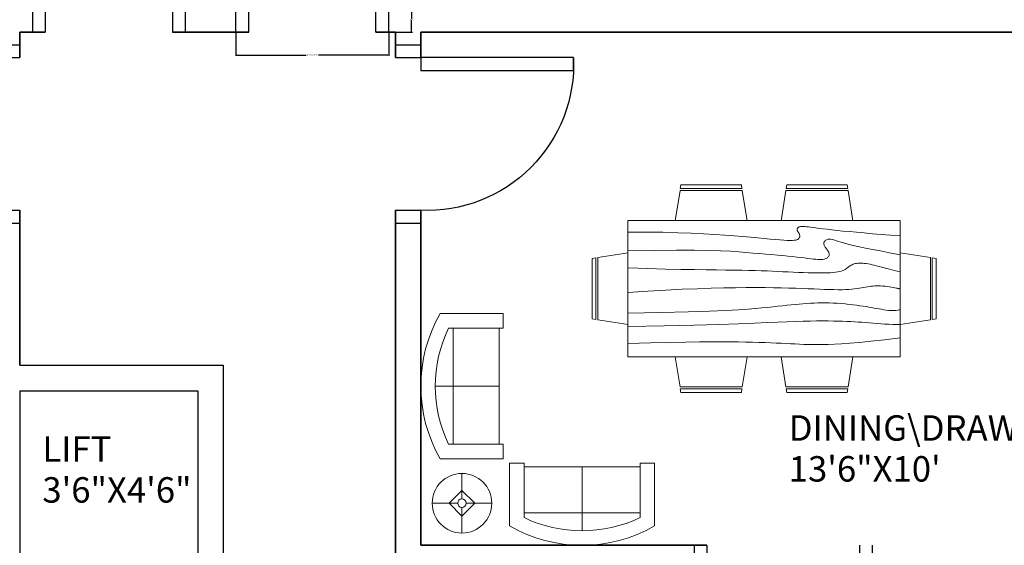
# Model space of a CAD drawing. Units: inches. Extents: x 4159 to 4826, y 299 to 1026.
# Tile 33 of 37: x 4453 to 4685, y 539 to 663. Entities that reach past the tile are written whole.
import ezdxf

# ---------------------------------------------------------------- set-up
doc = ezdxf.new("R2010")
doc.units = ezdxf.units.IN
for name, color, linetype, lineweight in [('A-ANNO-DIMS', 2, 'Continuous', 18), ('A-AREA-IDEN', 7, 'Continuous', 18), ('A-DOOR', 4, 'Continuous', 25), ('A-FLOR-EVTR', 6, 'Continuous', 25), ('A-FURN', 8, 'Continuous', 18), ('A-WALL', 7, 'Continuous', 35)]:
    doc.layers.add(name, color=color, linetype=linetype, lineweight=lineweight)
doc.styles.get("Standard").update_dxf_attribs({"font": 'arial.ttf'})
doc.dimstyles.get("Standard").update_dxf_attribs({"dimtxt": 0.18, "dimasz": 0.18, "dimexe": 0.18, "dimexo": 0.0625, "dimgap": 0.09, "dimtad": 0, "dimtih": 1, "dimtoh": 1, "dimdec": 4, "dimzin": 0, "dimdsep": 46, "dimtxsty": 'Standard', "dimcen": 0.09, "dimadec": 0, "dimazin": 0, "dimtfac": 1, "dimtdec": 4, "dimtofl": 0, "dimtmove": 0, "dimatfit": 3, "dimfxl": 1, "dimtolj": 1, "dimtzin": 0, "dimarcsym": 0})

# ---------------------------------------------------------------- blocks, each defined once
blk = doc.blocks.new('Sofa - Roundback Loveseat 5 ft.')
for p, q in [((0, -32.44198), (0, -5.99998)), ((-24, -33.99998), (-24, -11.46958)), ((24.00004, -33.99998), (24.00004, -11.46958)), ((-23.9998, -13.38178), (23.99986, -13.38178)), ((-24, -32.44198), (24.00004, -32.44198))]:
    blk.add_line(p, q)
for points in [[(-24, -33.99998), (-30, -33.99998), (-30, -7.99998)], [(30.00004, -7.99998), (30.00004, -33.99998), (24.00004, -33.99998)]]:
    blk.add_lwpolyline(points)
for centre, radius, start, end in [((0, -60.24998), 60.24998, 60.13715, 119.8628), ((0, -61.38438), 55.38444, 64.32083, 115.6792)]:
    blk.add_arc(centre, radius, start, end)
blk = doc.blocks.new('Dining Set - 36 x 72 in.')
for p, q in [((-22, 27.5), (-22.1562, 26.50042)), ((-5.8416, 26.5), (-22.1534, 26.5)), ((-22, 27.5), (-6, 27.5)), ((-5.8437, 26.49966), (-6, 27.5)), ((6, 27.5), (5.8438, 26.50042)), ((22.1584, 26.5), (5.8466, 26.5)), ((6, 27.5), (22, 27.5)), ((22.1563, 26.49966), (22, 27.5)), ((-22.2343, 26.00059), (-23.4847, 17.99762)), ((-22.2304, 26), (-5.7608, 26)), ((-4.5152, 17.99762), (-5.7655, 25.99926)), ((5.7657, 26.00059), (4.5153, 17.99762)), ((5.7696, 26), (22.2392, 26)), ((23.4848, 17.99762), (22.2345, 25.99926)), ((36, 18), (-36, 18)), ((-36, 18), (-36, -18)), ((36, -18), (36, 18)), ((-45.5, 8), (-44.5004, 8.15617)), ((-45.5, 8), (-45.5, -8)), ((-44.5, -8.15843), (-44.5, 8.15338)), ((-44.0006, 8.23428), (-35.9976, 9.48474)), ((-44, 8.23041), (-44, -8.23915)), ((44.0006, 8.23428), (35.9976, 9.48474)), ((44, 8.23041), (44, -8.23915)), ((44.5, -8.15843), (44.5, 8.15338)), ((45.5, 8), (44.5005, 8.15617)), ((45.5, 8), (45.5, -8)), ((-44.4997, -8.15631), (-45.5, -8)), ((-35.9976, -9.48476), (-43.9993, -8.2345)), ((35.9976, -9.48476), (43.9993, -8.2345)), ((44.4997, -8.15631), (45.5, -8)), ((-36, -18), (36, -18)), ((-22.2343, -26.0006), (-23.4847, -17.99762)), ((-4.5152, -17.99762), (-5.7655, -25.99928)), ((5.7657, -26.0006), (4.5153, -17.99762)), ((23.4848, -17.99762), (22.2345, -25.99928)), ((-22.2304, -26), (-5.7608, -26)), ((5.7696, -26), (22.2392, -26)), ((-22, -27.5), (-22.1562, -26.50044)), ((-5.8416, -26.5), (-22.1534, -26.5)), ((-22, -27.5), (-6, -27.5)), ((-5.8437, -26.49967), (-6, -27.5)), ((6, -27.5), (5.8438, -26.50044)), ((22.1584, -26.5), (5.8466, -26.5)), ((6, -27.5), (22, -27.5)), ((22.1563, -26.49967), (22, -27.5))]:
    blk.add_line(p, q)
for points in [[(-36, 15), (-31.1772, 14.97754), (-26.8079, 14.91406), (-22.8538, 14.81543), (-19.276, 14.6875), (-16.0362, 14.53613), (-13.0957, 14.36718), (-10.4159, 14.18652), (-7.9583, 14), (-5.6904, 13.81315), (-3.6035, 13.63021), (-1.6954, 13.45508), (0.0365, 13.29166), (1.5945, 13.14388), (2.9811, 13.01562), (4.1988, 12.9108), (5.25, 12.83333), (6.1393, 12.78613), (6.8802, 12.76823), (7.4883, 12.77767), (7.9792, 12.8125), (8.3685, 12.87077), (8.6719, 12.95052), (8.9049, 13.0498), (9.0833, 13.16666), (9.2205, 13.29899), (9.3216, 13.44401), (9.3895, 13.59879), (9.4271, 13.76041), (9.4373, 13.92594), (9.4232, 14.09245), (9.3875, 14.257), (9.3333, 14.41666), (9.2638, 14.56917), (9.1836, 14.71484), (9.0975, 14.85465), (9.0104, 14.98958), (8.9272, 15.1206), (8.8529, 15.2487), (8.7922, 15.37483), (8.75, 15.5), (8.7305, 15.62467), (8.7344, 15.74739), (8.7617, 15.86621), (8.8125, 15.97916), (8.8867, 16.08431), (8.9844, 16.17968), (9.1055, 16.26334), (9.25, 16.33333), (9.4189, 16.38802), (9.6172, 16.42708), (9.8506, 16.45052), (10.125, 16.45833), (10.4463, 16.45052), (10.8203, 16.42708), (11.2529, 16.38802), (11.75, 16.33333), (12.3184, 16.26318), (12.9694, 16.17838), (13.7151, 16.07991), (14.5677, 15.96875), (15.5395, 15.84586), (16.6426, 15.71224), (17.8893, 15.56884), (19.2917, 15.41666), (20.859, 15.25667), (22.5879, 15.08984), (24.4721, 14.91715), (26.5052, 14.73958), (28.6809, 14.5581), (30.9929, 14.3737), (33.4347, 14.18733), (36, 14)], [(-36, 10), (-28.9766, 10.14274), (-23.1725, 10.20442), (-18.4241, 10.19775), (-14.5677, 10.13541), (-11.4399, 10.03011), (-8.877, 9.89453), (-6.7154, 9.74137), (-4.7917, 9.58333), (-2.9698, 9.43082), (-1.2246, 9.28515), (0.4415, 9.14534), (2.026, 9.01041), (3.5266, 8.87939), (4.9408, 8.7513), (6.266, 8.62516), (7.5, 8.5), (8.6411, 8.37549), (9.6914, 8.2539), (10.6538, 8.13818), (11.5312, 8.03125), (12.3267, 7.93603), (13.043, 7.85547), (13.6831, 7.79248), (14.25, 7.75), (14.7471, 7.7303), (15.1797, 7.73307), (15.5537, 7.75732), (15.875, 7.80208), (16.1494, 7.86637), (16.3828, 7.94922), (16.5811, 8.04964), (16.75, 8.16666), (16.8944, 8.29915), (17.0143, 8.44531), (17.1089, 8.60319), (17.1771, 8.77083), (17.218, 8.94629), (17.2305, 9.1276), (17.2137, 9.31282), (17.1667, 9.5), (17.0895, 9.6875), (16.987, 9.875), (16.8649, 10.0625), (16.7292, 10.25), (16.5856, 10.4375), (16.4401, 10.625), (16.2985, 10.8125), (16.1667, 11), (16.05, 11.18733), (15.9518, 11.3737), (15.8752, 11.5581), (15.8229, 11.73958), (15.798, 11.91715), (15.8034, 12.08984), (15.842, 12.25667), (15.9167, 12.41666), (16.0295, 12.56836), (16.1784, 12.70833), (16.3605, 12.83268), (16.5729, 12.9375), (16.8127, 13.01888), (17.0768, 13.07291), (17.3625, 13.0957), (17.6667, 13.08333), (17.9894, 13.03312), (18.3418, 12.94726), (18.7382, 12.82918), (19.1927, 12.68229), (19.7195, 12.51001), (20.3327, 12.31575), (21.0465, 12.10294), (21.875, 11.875), (22.8357, 11.63354), (23.959, 11.37304), (25.2786, 11.08618), (26.8282, 10.76562), (28.6414, 10.40405), (30.752, 9.99414), (33.1936, 9.52856), (36, 9)], [(-36, 5.5), (-30.7157, 5.3348), (-26.069, 5.20963), (-21.9946, 5.11767), (-18.4271, 5.05208), (-15.3009, 5.00602), (-12.5508, 4.97265), (-10.1112, 4.94515), (-7.9167, 4.91666), (-5.909, 4.88167), (-4.0586, 4.83984), (-2.3429, 4.79215), (-0.7396, 4.73958), (0.7739, 4.6831), (2.22, 4.6237), (3.6213, 4.56233), (5, 4.5), (6.373, 4.43782), (7.7344, 4.3776), (9.0723, 4.32129), (10.375, 4.27083), (11.6309, 4.22819), (12.8281, 4.19531), (13.9551, 4.17415), (15, 4.16666), (15.954, 4.17448), (16.819, 4.19791), (17.6001, 4.23698), (18.3021, 4.29166), (18.9299, 4.36198), (19.4883, 4.44791), (19.9823, 4.54948), (20.4167, 4.66666), (20.7969, 4.79899), (21.1302, 4.94401), (21.4245, 5.09879), (21.6875, 5.26041), (21.9271, 5.42594), (22.1511, 5.59245), (22.3672, 5.757), (22.5834, 5.91666), (22.8065, 6.06868), (23.0404, 6.21093), (23.2879, 6.34147), (23.5521, 6.45833), (23.8358, 6.55957), (24.142, 6.64323), (24.4735, 6.70735), (24.8334, 6.75), (25.2235, 6.76969), (25.642, 6.76692), (26.0858, 6.74267), (26.5521, 6.69791), (27.0379, 6.63362), (27.5404, 6.55078), (28.0565, 6.45036), (28.5834, 6.33333), (29.1242, 6.19987), (29.7071, 6.04687), (30.3661, 5.87044), (31.1354, 5.66666), (32.0493, 5.43164), (33.142, 5.16146), (34.4475, 4.85221), (36, 4.5)], [(-36, -1), (-30.7915, -0.6591), (-26.0195, -0.38216), (-21.6519, -0.16284), (-17.6563, 0.00521), (-14.0005, 0.12833), (-10.6523, 0.21289), (-7.5796, 0.26522), (-4.75, 0.29166), (-2.134, 0.29793), (0.2878, 0.28711), (2.5317, 0.26163), (4.6146, 0.22396), (6.5529, 0.17651), (8.3633, 0.12174), (10.0623, 0.06209), (11.6667, 0), (13.1899, -0.06201), (14.6341, -0.1211), (15.9982, -0.17432), (17.2813, -0.21875), (18.4823, -0.25147), (19.6003, -0.26953), (20.6343, -0.27002), (21.5834, -0.25), (22.4481, -0.20768), (23.2357, -0.14584), (23.9549, -0.06836), (24.6146, 0.02083), (25.2235, 0.11784), (25.7904, 0.21875), (26.3241, 0.31966), (26.8334, 0.41666), (27.3265, 0.50618), (27.8099, 0.58593), (28.2894, 0.65397), (28.7709, 0.70833), (29.2601, 0.74707), (29.763, 0.76823), (30.2855, 0.76985), (30.8334, 0.75), (31.4088, 0.70784), (31.9994, 0.64713), (32.589, 0.57275), (33.1615, 0.48958), (33.7008, 0.4025), (34.1908, 0.3164), (34.6153, 0.23616), (34.9584, 0.16666), (35.2099, 0.11165), (35.3848, 0.07031), (35.504, 0.04069), (35.5886, 0.02083), (35.6594, 0.00879), (35.7377, 0.0026), (35.8442, 0.00032), (36, 0)], [(-36, -6.5), (-27.1843, -6.31267), (-20.084, -6.1263), (-14.469, -5.9419), (-10.1094, -5.76042), (-6.7752, -5.58285), (-4.2363, -5.41016), (-2.2629, -5.24333), (-0.625, -5.08334), (0.8708, -4.93099), (2.2715, -4.78646), (3.5872, -4.64974), (4.8281, -4.52084), (6.0046, -4.39974), (7.127, -4.28646), (8.2053, -4.18099), (9.25, -4.08334), (10.2705, -3.99382), (11.2734, -3.91407), (12.2647, -3.84603), (13.25, -3.79167), (14.2354, -3.75293), (15.2266, -3.73177), (16.2295, -3.73015), (17.25, -3.75), (18.2912, -3.79248), (19.3451, -3.85547), (20.4009, -3.93604), (21.4479, -4.03125), (22.4754, -4.13819), (23.4727, -4.25391), (24.4289, -4.37549), (25.3334, -4.5), (26.1785, -4.62492), (26.9694, -4.74935), (27.7145, -4.87281), (28.4219, -4.99479), (29.1, -5.11483), (29.7572, -5.23242), (30.4016, -5.34709), (31.0417, -5.45834), (31.6837, -5.56437), (32.3262, -5.65821), (32.9658, -5.73153), (33.599, -5.77604), (34.2224, -5.78345), (34.8327, -5.74545), (35.4264, -5.65373), (36, -5.5)], [(-36, -10), (-26.4022, -9.81299), (-18.4675, -9.62891), (-11.9839, -9.45069), (-6.7396, -9.28125), (-2.5226, -9.12354), (0.8789, -8.98047), (3.6769, -8.85498), (6.0833, -8.75), (8.2767, -8.66765), (10.3021, -8.60677), (12.1712, -8.56543), (13.8958, -8.54167), (15.4876, -8.53353), (16.9583, -8.53907), (18.3197, -8.55632), (19.5834, -8.58334), (20.7616, -8.61841), (21.8685, -8.66081), (22.9188, -8.71004), (23.9271, -8.76563), (24.9081, -8.82707), (25.8763, -8.89388), (26.8465, -8.96558), (27.8334, -9.04167), (28.8474, -9.12118), (29.8828, -9.20117), (30.93, -9.27824), (31.9792, -9.34896), (33.0205, -9.40991), (34.0443, -9.45768), (35.0407, -9.48885), (36, -9.5)], [(-36, -14.5), (-30.0881, -14.33513), (-25.0332, -14.21224), (-20.7312, -14.12647), (-17.0781, -14.07292), (-13.97, -14.04671), (-11.3027, -14.04297), (-8.9724, -14.05681), (-6.875, -14.08334), (-4.9224, -14.11833), (-3.0905, -14.16016), (-1.3709, -14.20785), (0.2448, -14.26042), (1.7647, -14.3169), (3.1973, -14.3763), (4.5507, -14.43767), (5.8333, -14.5), (7.0554, -14.5621), (8.235, -14.62175), (9.3922, -14.67652), (10.5469, -14.72396), (11.7192, -14.76164), (12.929, -14.78711), (14.1965, -14.79794), (15.5417, -14.79167), (16.9933, -14.76424), (18.6152, -14.70508), (20.4804, -14.60197), (22.6615, -14.44271), (25.2312, -14.21509), (28.2624, -13.9069), (31.8277, -13.50594), (36, -13)]]:
    blk.add_lwpolyline(points)
blk = doc.blocks.new('Lamp - Table')
for p, q in [((0, 7), (0, 1)), ((0, 3), (-3, 0)), ((3, 0), (0, 3)), ((-1, 0), (-7, 0)), ((-3, 0), (0, -3)), ((0, -3), (3, 0)), ((1, 0), (7, 0)), ((0, -1), (0, -7))]:
    blk.add_line(p, q)
for radius in [7, 1]:
    blk.add_circle((0, 0), radius)
blk = doc.blocks.new('DOOR-SWING-36IN')
blk.add_lwpolyline([(0, 0), (-3, 0), (-3, 36), (0, 36)], close=True)
blk.add_arc((-1.5, 1.5), 34.53, 87.5104, 182.4896)
blk = doc.blocks.new('DOOR-FRAME-36IN')
for p, q in [((0, 6), (0, 0)), ((3, 6), (3, 0)), ((39, 6), (39, 0)), ((42, 6), (42, 0))]:
    blk.add_line(p, q)
blk = doc.blocks.new('DOOR-FRAME-30IN')
for p, q in [((0, 6), (0, 0)), ((3, 6), (3, 0)), ((33, 6), (33, 0)), ((36, 6), (36, 0))]:
    blk.add_line(p, q)
blk = doc.blocks.new('*D21')
at = {"layer": 'A-ANNO-DIMS', "color": 0, "lineweight": -2, "transparency": 16777216}
for p, q in [((4504.31, 660.19), (4504.31, 654.67)), ((4540.31, 660.19), (4540.31, 654.67)), ((4504.49, 654.85), (4520.85, 654.85)), ((4540.13, 654.85), (4523.77, 654.85))]:
    blk.add_line(p, q, dxfattribs=at)
at = {"layer": 'A-ANNO-DIMS', "color": 0, "transparency": 16777216}
for points in [[(4504.49, 654.88), (4504.49, 654.82), (4504.31, 654.85)], [(4540.13, 654.88), (4540.13, 654.82), (4540.31, 654.85)]]:
    blk.add_solid(points, dxfattribs=at)
at = {"layer": 'Defpoints', "color": 0, "transparency": 16777216}
for p in [(4504.31, 660.25), (4540.31, 660.25), (4504.31, 654.85)]:
    blk.add_point(p, dxfattribs=at)
at = {"layer": 'A-ANNO-DIMS', "color": 0, "transparency": 16777216, "insert": (4522.31, 654.85), "char_height": 0.18, "attachment_point": 5}
blk.add_mtext('\\A1;ENTRY FRAME 36 TYP.', dxfattribs=at)
blk = doc.blocks.new('*D22')
at = {"layer": 'A-ANNO-DIMS', "color": 0, "lineweight": -2, "transparency": 16777216}
for p, q in [((4540.37, 666.25), (4545.89, 666.25)), ((4545.71, 666.07), (4545.71, 663.44)), ((4545.71, 660.43), (4545.71, 663.07)), ((4540.37, 660.25), (4545.89, 660.25))]:
    blk.add_line(p, q, dxfattribs=at)
at = {"layer": 'A-ANNO-DIMS', "color": 0, "transparency": 16777216}
for points in [[(4545.68, 666.07), (4545.74, 666.07), (4545.71, 666.25)], [(4545.68, 660.43), (4545.74, 660.43), (4545.71, 660.25)]]:
    blk.add_solid(points, dxfattribs=at)
at = {"layer": 'Defpoints', "color": 0, "transparency": 16777216}
for p in [(4540.31, 666.25), (4540.31, 660.25), (4545.71, 660.25)]:
    blk.add_point(p, dxfattribs=at)
at = {"layer": 'A-ANNO-DIMS', "color": 0, "transparency": 16777216, "insert": (4545.71, 663.25), "char_height": 0.18, "attachment_point": 5}
blk.add_mtext('\\A1;6 TYP.', dxfattribs=at)

msp = doc.modelspace()

# ---------------------------------------------------------------- linework, layer by layer
at = {"layer": 'A-FLOR-EVTR'}
for p, q in [((4453.31, 581.713), (4501.31, 581.713)), ((4501.31, 581.713), (4501.31, 515.713)), ((4453.31, 575.713), (4495.31, 575.713)), ((4453.31, 575.713), (4453.31, 521.713)), ((4495.31, 575.713), (4495.31, 521.713))]:
    msp.add_line(p, q, dxfattribs=at)
at = {"layer": 'A-WALL'}
for p, q in [((4453.31, 660.254), (4453.31, 654.254)), ((4459.31, 660.254), (4453.31, 660.254)), ((4507.31, 660.254), (4489.31, 660.254)), ((4541.889, 660.254), (4537.31, 660.254)), ((4541.889, 660.254), (4541.889, 654.254)), ((4741.31, 660.254), (4547.889, 660.254)), ((4547.889, 660.254), (4547.889, 654.254)), ((4453.31, 618.254), (4453.31, 581.713)), ((4541.889, 618.254), (4541.889, 401.254)), ((4547.889, 618.254), (4547.889, 539.254)), ((4615.31, 539.254), (4547.889, 539.254))]:
    msp.add_line(p, q, dxfattribs=at)

# ---------------------------------------------------------------- block references
at = {"layer": 'A-DOOR'}
for name, p in [('DOOR-FRAME-30IN', (4456.31, 660.254)), ('DOOR-FRAME-36IN', (4612.31, 533.254))]:
    msp.add_blockref(name, p, dxfattribs=at)
for name, p, rotation in [('DOOR-FRAME-30IN', (4540.31, 666.254), 180), ('DOOR-FRAME-36IN', (4453.31, 615.254), 90.0000000000003), ('DOOR-FRAME-36IN', (4547.889, 615.254), 90.00000000000276)]:
    msp.add_blockref(name, p, dxfattribs=dict(at, rotation=rotation))
at = {"layer": 'A-DOOR', "extrusion": (0, 0, -1), "zscale": -1, "rotation": 90.00000000000288}
msp.add_blockref('DOOR-SWING-36IN', (-4547.889, 654.254), dxfattribs=at)
at = {"layer": 'A-FURN'}
for name, p, xscale, yscale, zscale in [('Dining Set - 36 x 72 in.', (4628.826, 599.771), 0.8913588978043845, 0.8913588978043845, 0.8913588978043845), ('Lamp - Table', (4557.593, 549.173), 1.003057144141322, 1.003057144141322, 1.003057144141322)]:
    msp.add_blockref(name, p, dxfattribs=dict(at, xscale=xscale, yscale=yscale, zscale=zscale))
at = {"layer": 'A-FURN', "xscale": 0.5700533147329089, "yscale": 0.5700533147329089, "zscale": 0.5700533147329089}
for p, rotation in [((4547.889, 576.781), 90), ((4585.903, 539.254), 180)]:
    msp.add_blockref('Sofa - Roundback Loveseat 5 ft.', p, dxfattribs=dict(at, rotation=rotation))

# ---------------------------------------------------------------- texts
at = {"layer": 'A-AREA-IDEN'}
for s, p in [('DINING\\DRAWING', (4634.632, 563.924)), ('LIFT', (4458.652, 558.954)), ('13\'6"X10\'', (4634.632, 554.286)), ('3\'6"X4\'6"', (4458.652, 549.315))]:
    msp.add_text(s, height=6, dxfattribs=at).set_placement(p)

# ---------------------------------------------------------------- dimensions: what is measured, and where the dimension line sits
at = {"layer": 'A-ANNO-DIMS'}
for base, p1, p2, angle, text, picture, middle in [((4545.71, 660.254), (4540.31, 666.254), (4540.31, 660.254), 270, '<> TYP.', '*D22', (4545.71, 663.254)), ((4504.31, 654.854), (4540.31, 660.254), (4504.31, 660.254), 180, 'ENTRY FRAME <> TYP.', '*D21', (4522.31, 654.854))]:
    dim = msp.add_linear_dim(base=base, p1=p1, p2=p2, angle=angle, text=text, dimstyle='Standard', override={"dimdec": 0, "dimlfac": 1, "dimrnd": 0, "dimzin": 0, "dimdsep": 46, "dimlunit": 2}, dxfattribs=at)
    dim.commit()
    dim.dimension.update_dxf_attribs({"geometry": picture, "text_midpoint": middle})

doc.saveas('drawing.dxf')
